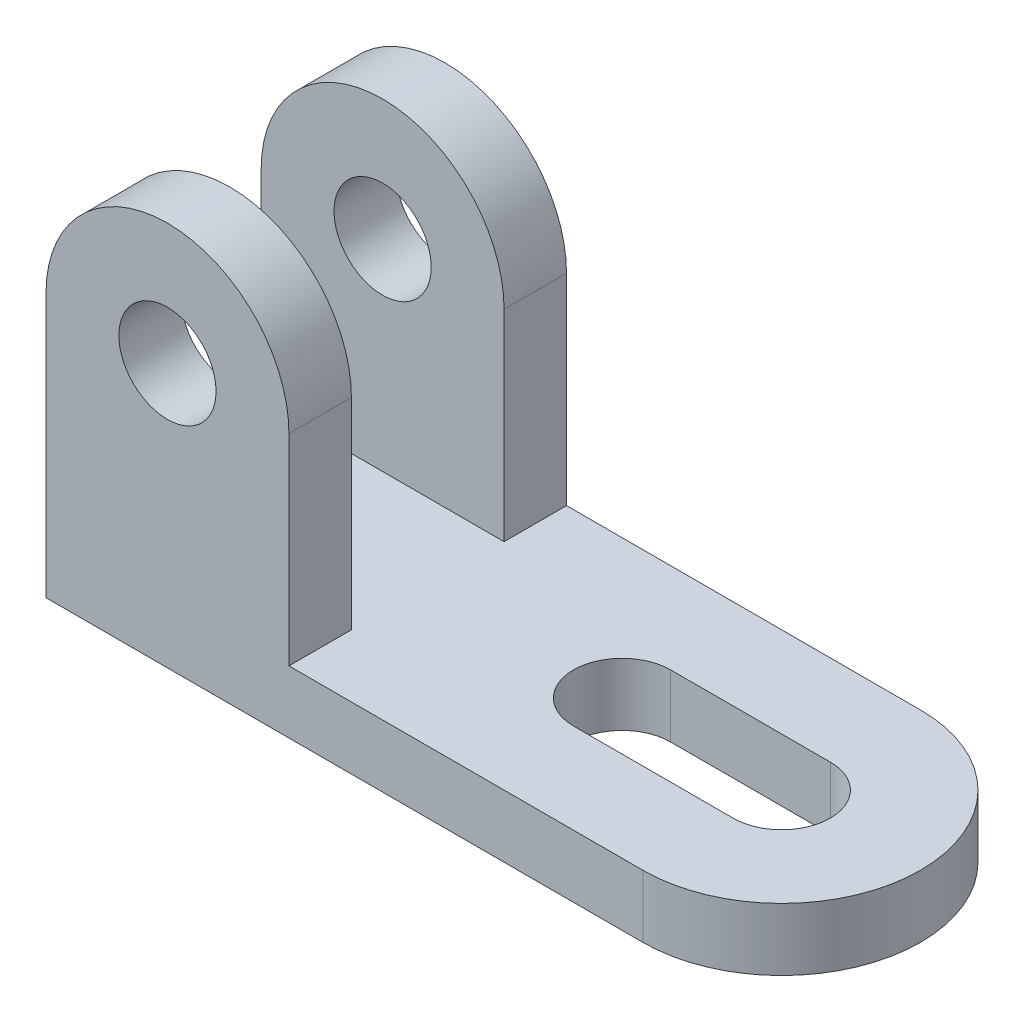
ISO-10303-21;
HEADER;
FILE_DESCRIPTION(('STEP AP214'),'2;1');
FILE_NAME('part.step','',(''),(''),'','','');
FILE_SCHEMA(('AUTOMOTIVE_DESIGN { 1 0 10303 214 1 1 1 1 }'));
ENDSEC;
DATA;
#1=APPLICATION_CONTEXT('core data for automotive mechanical design processes');
#2=APPLICATION_PROTOCOL_DEFINITION('international standard','automotive_design',2000,#1);
#3=PRODUCT_CONTEXT('',#1,'mechanical');
#4=PRODUCT('Part','Part','',(#3));
#5=PRODUCT_RELATED_PRODUCT_CATEGORY('part','',(#4));
#6=PRODUCT_DEFINITION_FORMATION('','',#4);
#7=PRODUCT_DEFINITION_CONTEXT('part definition',#1,'design');
#8=PRODUCT_DEFINITION('design','',#6,#7);
#9=PRODUCT_DEFINITION_SHAPE('','',#8);
#10=(LENGTH_UNIT() NAMED_UNIT(*) SI_UNIT(.MILLI.,.METRE.));
#11=(NAMED_UNIT(*) PLANE_ANGLE_UNIT() SI_UNIT($,.RADIAN.));
#12=(NAMED_UNIT(*) SI_UNIT($,.STERADIAN.) SOLID_ANGLE_UNIT());
#13=UNCERTAINTY_MEASURE_WITH_UNIT(LENGTH_MEASURE(1.E-05),#10,'distance_accuracy_value','');
#14=(GEOMETRIC_REPRESENTATION_CONTEXT(3) GLOBAL_UNCERTAINTY_ASSIGNED_CONTEXT((#13)) GLOBAL_UNIT_ASSIGNED_CONTEXT((#10,
#11,#12)) REPRESENTATION_CONTEXT('',''));
#15=CARTESIAN_POINT('',(0.,0.,0.));
#16=DIRECTION('',(0.,0.,1.));
#17=DIRECTION('',(1.,0.,0.));
#18=AXIS2_PLACEMENT_3D('',#15,#16,#17);
#19=CARTESIAN_POINT('',(86.,9.,0.));
#20=DIRECTION('',(0.,1.,0.));
#21=DIRECTION('',(0.,0.,1.));
#22=AXIS2_PLACEMENT_3D('',#19,#20,#21);
#23=PLANE('',#22);
#24=DIRECTION('',(0.,0.,-1.));
#25=VECTOR('',#24,1.);
#26=CARTESIAN_POINT('',(35.,9.,-11.));
#27=LINE('',#26,#25);
#28=CARTESIAN_POINT('',(35.,9.,-11.));
#29=VERTEX_POINT('',#28);
#30=CARTESIAN_POINT('',(35.,9.,-20.));
#31=VERTEX_POINT('',#30);
#32=EDGE_CURVE('E57',#29,#31,#27,.T.);
#33=ORIENTED_EDGE('',*,*,#32,.F.);
#34=DIRECTION('',(-1.,0.,0.));
#35=VECTOR('',#34,1.);
#36=CARTESIAN_POINT('',(0.,9.,-11.));
#37=LINE('',#36,#35);
#38=CARTESIAN_POINT('',(0.,9.,-11.));
#39=VERTEX_POINT('',#38);
#40=EDGE_CURVE('E164',#29,#39,#37,.T.);
#41=ORIENTED_EDGE('',*,*,#40,.T.);
#42=DIRECTION('',(0.,0.,1.));
#43=VECTOR('',#42,1.);
#44=CARTESIAN_POINT('',(0.,9.,-20.));
#45=LINE('',#44,#43);
#46=CARTESIAN_POINT('',(0.,9.,11.));
#47=VERTEX_POINT('',#46);
#48=EDGE_CURVE('E163',#39,#47,#45,.T.);
#49=ORIENTED_EDGE('',*,*,#48,.T.);
#50=DIRECTION('',(-1.,0.,0.));
#51=VECTOR('',#50,1.);
#52=CARTESIAN_POINT('',(0.,9.,11.));
#53=LINE('',#52,#51);
#54=CARTESIAN_POINT('',(35.,9.,11.));
#55=VERTEX_POINT('',#54);
#56=EDGE_CURVE('E187',#55,#47,#53,.T.);
#57=ORIENTED_EDGE('',*,*,#56,.F.);
#58=DIRECTION('',(0.,0.,1.));
#59=VECTOR('',#58,1.);
#60=CARTESIAN_POINT('',(35.,9.,11.));
#61=LINE('',#60,#59);
#62=CARTESIAN_POINT('',(35.,9.,20.));
#63=VERTEX_POINT('',#62);
#64=EDGE_CURVE('E206',#55,#63,#61,.T.);
#65=ORIENTED_EDGE('',*,*,#64,.T.);
#66=DIRECTION('',(1.,0.,0.));
#67=VECTOR('',#66,1.);
#68=CARTESIAN_POINT('',(86.,9.,20.));
#69=LINE('',#68,#67);
#70=CARTESIAN_POINT('',(86.,9.,20.));
#71=VERTEX_POINT('',#70);
#72=EDGE_CURVE('E241',#63,#71,#69,.T.);
#73=ORIENTED_EDGE('',*,*,#72,.T.);
#74=CARTESIAN_POINT('',(86.,9.,0.));
#75=DIRECTION('',(0.,1.,0.));
#76=DIRECTION('',(0.,0.,1.));
#77=AXIS2_PLACEMENT_3D('',#74,#75,#76);
#78=CIRCLE('',#77,20.);
#79=CARTESIAN_POINT('',(86.,9.,-20.));
#80=VERTEX_POINT('',#79);
#81=EDGE_CURVE('E243',#71,#80,#78,.T.);
#82=ORIENTED_EDGE('',*,*,#81,.T.);
#83=DIRECTION('',(-1.,0.,0.));
#84=VECTOR('',#83,1.);
#85=CARTESIAN_POINT('',(86.,9.,-20.));
#86=LINE('',#85,#84);
#87=EDGE_CURVE('E64',#80,#31,#86,.T.);
#88=ORIENTED_EDGE('',*,*,#87,.T.);
#89=EDGE_LOOP('',(#33,#41,#49,#57,#65,#73,#82,#88));
#90=FACE_BOUND('',#89,.T.);
#91=DIRECTION('',(-1.,0.,0.));
#92=VECTOR('',#91,1.);
#93=CARTESIAN_POINT('',(86.,9.,-7.));
#94=LINE('',#93,#92);
#95=CARTESIAN_POINT('',(86.,9.,-7.));
#96=VERTEX_POINT('',#95);
#97=CARTESIAN_POINT('',(63.,9.,-7.));
#98=VERTEX_POINT('',#97);
#99=EDGE_CURVE('E213',#96,#98,#94,.T.);
#100=ORIENTED_EDGE('',*,*,#99,.F.);
#101=CARTESIAN_POINT('',(86.,9.,0.));
#102=DIRECTION('',(0.,1.,0.));
#103=DIRECTION('',(0.,0.,1.));
#104=AXIS2_PLACEMENT_3D('',#101,#102,#103);
#105=CIRCLE('',#104,7.);
#106=CARTESIAN_POINT('',(86.,9.,7.));
#107=VERTEX_POINT('',#106);
#108=EDGE_CURVE('E211',#107,#96,#105,.T.);
#109=ORIENTED_EDGE('',*,*,#108,.F.);
#110=DIRECTION('',(1.,0.,0.));
#111=VECTOR('',#110,1.);
#112=CARTESIAN_POINT('',(86.,9.,7.));
#113=LINE('',#112,#111);
#114=CARTESIAN_POINT('',(63.,9.,7.));
#115=VERTEX_POINT('',#114);
#116=EDGE_CURVE('E218',#115,#107,#113,.T.);
#117=ORIENTED_EDGE('',*,*,#116,.F.);
#118=CARTESIAN_POINT('',(63.,9.,0.));
#119=DIRECTION('',(0.,1.,0.));
#120=DIRECTION('',(0.,0.,1.));
#121=AXIS2_PLACEMENT_3D('',#118,#119,#120);
#122=CIRCLE('',#121,7.);
#123=EDGE_CURVE('E216',#98,#115,#122,.T.);
#124=ORIENTED_EDGE('',*,*,#123,.F.);
#125=EDGE_LOOP('',(#100,#109,#117,#124));
#126=FACE_BOUND('',#125,.T.);
#127=ADVANCED_FACE('F41',(#90,#126),#23,.T.);
#128=CARTESIAN_POINT('',(86.,0.,0.));
#129=DIRECTION('',(0.,1.,0.));
#130=DIRECTION('',(0.,0.,1.));
#131=AXIS2_PLACEMENT_3D('',#128,#129,#130);
#132=PLANE('',#131);
#133=DIRECTION('',(1.,0.,0.));
#134=VECTOR('',#133,1.);
#135=CARTESIAN_POINT('',(86.,0.,20.));
#136=LINE('',#135,#134);
#137=CARTESIAN_POINT('',(0.,0.,20.));
#138=VERTEX_POINT('',#137);
#139=CARTESIAN_POINT('',(86.,0.,20.));
#140=VERTEX_POINT('',#139);
#141=EDGE_CURVE('E244',#138,#140,#136,.T.);
#142=ORIENTED_EDGE('',*,*,#141,.F.);
#143=DIRECTION('',(0.,0.,1.));
#144=VECTOR('',#143,1.);
#145=CARTESIAN_POINT('',(0.,0.,-20.));
#146=LINE('',#145,#144);
#147=CARTESIAN_POINT('',(0.,0.,-20.));
#148=VERTEX_POINT('',#147);
#149=EDGE_CURVE('E242',#148,#138,#146,.T.);
#150=ORIENTED_EDGE('',*,*,#149,.F.);
#151=DIRECTION('',(-1.,0.,0.));
#152=VECTOR('',#151,1.);
#153=CARTESIAN_POINT('',(86.,0.,-20.));
#154=LINE('',#153,#152);
#155=CARTESIAN_POINT('',(86.,0.,-20.));
#156=VERTEX_POINT('',#155);
#157=EDGE_CURVE('E255',#156,#148,#154,.T.);
#158=ORIENTED_EDGE('',*,*,#157,.F.);
#159=CARTESIAN_POINT('',(86.,0.,0.));
#160=DIRECTION('',(0.,1.,0.));
#161=DIRECTION('',(0.,0.,1.));
#162=AXIS2_PLACEMENT_3D('',#159,#160,#161);
#163=CIRCLE('',#162,20.);
#164=EDGE_CURVE('E252',#140,#156,#163,.T.);
#165=ORIENTED_EDGE('',*,*,#164,.F.);
#166=EDGE_LOOP('',(#142,#150,#158,#165));
#167=FACE_BOUND('',#166,.T.);
#168=CARTESIAN_POINT('',(86.,0.,0.));
#169=DIRECTION('',(0.,1.,0.));
#170=DIRECTION('',(0.,0.,1.));
#171=AXIS2_PLACEMENT_3D('',#168,#169,#170);
#172=CIRCLE('',#171,7.);
#173=CARTESIAN_POINT('',(86.,0.,7.));
#174=VERTEX_POINT('',#173);
#175=CARTESIAN_POINT('',(86.,0.,-7.));
#176=VERTEX_POINT('',#175);
#177=EDGE_CURVE('E202',#174,#176,#172,.T.);
#178=ORIENTED_EDGE('',*,*,#177,.T.);
#179=DIRECTION('',(-1.,0.,0.));
#180=VECTOR('',#179,1.);
#181=CARTESIAN_POINT('',(86.,0.,-7.));
#182=LINE('',#181,#180);
#183=CARTESIAN_POINT('',(63.,0.,-7.));
#184=VERTEX_POINT('',#183);
#185=EDGE_CURVE('E221',#176,#184,#182,.T.);
#186=ORIENTED_EDGE('',*,*,#185,.T.);
#187=CARTESIAN_POINT('',(63.,0.,0.));
#188=DIRECTION('',(0.,1.,0.));
#189=DIRECTION('',(0.,0.,1.));
#190=AXIS2_PLACEMENT_3D('',#187,#188,#189);
#191=CIRCLE('',#190,7.);
#192=CARTESIAN_POINT('',(63.,0.,7.));
#193=VERTEX_POINT('',#192);
#194=EDGE_CURVE('E226',#184,#193,#191,.T.);
#195=ORIENTED_EDGE('',*,*,#194,.T.);
#196=DIRECTION('',(1.,0.,0.));
#197=VECTOR('',#196,1.);
#198=CARTESIAN_POINT('',(86.,0.,7.));
#199=LINE('',#198,#197);
#200=EDGE_CURVE('E212',#193,#174,#199,.T.);
#201=ORIENTED_EDGE('',*,*,#200,.T.);
#202=EDGE_LOOP('',(#178,#186,#195,#201));
#203=FACE_BOUND('',#202,.T.);
#204=ADVANCED_FACE('F271',(#167,#203),#132,.F.);
#205=CARTESIAN_POINT('',(86.,9.,20.));
#206=DIRECTION('',(0.,0.,-1.));
#207=DIRECTION('',(-1.,0.,0.));
#208=AXIS2_PLACEMENT_3D('',#205,#206,#207);
#209=PLANE('',#208);
#210=ORIENTED_EDGE('',*,*,#141,.T.);
#211=DIRECTION('',(0.,-1.,0.));
#212=VECTOR('',#211,1.);
#213=CARTESIAN_POINT('',(86.,9.,20.));
#214=LINE('',#213,#212);
#215=EDGE_CURVE('E11',#71,#140,#214,.T.);
#216=ORIENTED_EDGE('',*,*,#215,.F.);
#217=ORIENTED_EDGE('',*,*,#72,.F.);
#218=DIRECTION('',(0.,-1.,0.));
#219=VECTOR('',#218,1.);
#220=CARTESIAN_POINT('',(35.,0.,20.));
#221=LINE('',#220,#219);
#222=CARTESIAN_POINT('',(35.,38.,20.));
#223=VERTEX_POINT('',#222);
#224=EDGE_CURVE('E183',#223,#63,#221,.T.);
#225=ORIENTED_EDGE('',*,*,#224,.F.);
#226=CARTESIAN_POINT('',(17.5,38.,20.));
#227=DIRECTION('',(0.,0.,1.));
#228=DIRECTION('',(1.,0.,0.));
#229=AXIS2_PLACEMENT_3D('',#226,#227,#228);
#230=CIRCLE('',#229,17.5);
#231=CARTESIAN_POINT('',(0.,38.,20.));
#232=VERTEX_POINT('',#231);
#233=EDGE_CURVE('E196',#232,#223,#230,.F.);
#234=ORIENTED_EDGE('',*,*,#233,.F.);
#235=DIRECTION('',(0.,-1.,0.));
#236=VECTOR('',#235,1.);
#237=CARTESIAN_POINT('',(0.,9.,20.));
#238=LINE('',#237,#236);
#239=EDGE_CURVE('E247',#232,#138,#238,.T.);
#240=ORIENTED_EDGE('',*,*,#239,.T.);
#241=EDGE_LOOP('',(#210,#216,#217,#225,#234,#240));
#242=FACE_BOUND('',#241,.T.);
#243=CARTESIAN_POINT('',(17.5,38.,20.));
#244=DIRECTION('',(0.,0.,1.));
#245=DIRECTION('',(1.,0.,0.));
#246=AXIS2_PLACEMENT_3D('',#243,#244,#245);
#247=CIRCLE('',#246,7.);
#248=CARTESIAN_POINT('',(24.5,38.,20.));
#249=VERTEX_POINT('',#248);
#250=EDGE_CURVE('E155',#249,#249,#247,.T.);
#251=ORIENTED_EDGE('',*,*,#250,.F.);
#252=EDGE_LOOP('',(#251));
#253=FACE_BOUND('',#252,.T.);
#254=ADVANCED_FACE('F43',(#242,#253),#209,.F.);
#255=CARTESIAN_POINT('',(86.,9.,0.));
#256=DIRECTION('',(0.,-1.,0.));
#257=DIRECTION('',(0.,0.,-1.));
#258=AXIS2_PLACEMENT_3D('',#255,#256,#257);
#259=CYLINDRICAL_SURFACE('',#258,20.);
#260=ORIENTED_EDGE('',*,*,#164,.T.);
#261=DIRECTION('',(0.,-1.,0.));
#262=VECTOR('',#261,1.);
#263=CARTESIAN_POINT('',(86.,9.,-20.));
#264=LINE('',#263,#262);
#265=EDGE_CURVE('E47',#80,#156,#264,.T.);
#266=ORIENTED_EDGE('',*,*,#265,.F.);
#267=ORIENTED_EDGE('',*,*,#81,.F.);
#268=ORIENTED_EDGE('',*,*,#215,.T.);
#269=EDGE_LOOP('',(#260,#266,#267,#268));
#270=FACE_BOUND('',#269,.T.);
#271=ADVANCED_FACE('F320',(#270),#259,.T.);
#272=CARTESIAN_POINT('',(86.,9.,-20.));
#273=DIRECTION('',(0.,0.,1.));
#274=DIRECTION('',(1.,0.,0.));
#275=AXIS2_PLACEMENT_3D('',#272,#273,#274);
#276=PLANE('',#275);
#277=ORIENTED_EDGE('',*,*,#157,.T.);
#278=DIRECTION('',(0.,-1.,0.));
#279=VECTOR('',#278,1.);
#280=CARTESIAN_POINT('',(0.,9.,-20.));
#281=LINE('',#280,#279);
#282=CARTESIAN_POINT('',(0.,38.,-20.));
#283=VERTEX_POINT('',#282);
#284=EDGE_CURVE('E259',#283,#148,#281,.T.);
#285=ORIENTED_EDGE('',*,*,#284,.F.);
#286=CARTESIAN_POINT('',(17.5,38.,-20.));
#287=DIRECTION('',(0.,0.,1.));
#288=DIRECTION('',(1.,0.,0.));
#289=AXIS2_PLACEMENT_3D('',#286,#287,#288);
#290=CIRCLE('',#289,17.5);
#291=CARTESIAN_POINT('',(35.,38.,-20.));
#292=VERTEX_POINT('',#291);
#293=EDGE_CURVE('E146',#283,#292,#290,.F.);
#294=ORIENTED_EDGE('',*,*,#293,.T.);
#295=DIRECTION('',(0.,-1.,0.));
#296=VECTOR('',#295,1.);
#297=CARTESIAN_POINT('',(35.,0.,-20.));
#298=LINE('',#297,#296);
#299=EDGE_CURVE('E176',#292,#31,#298,.T.);
#300=ORIENTED_EDGE('',*,*,#299,.T.);
#301=ORIENTED_EDGE('',*,*,#87,.F.);
#302=ORIENTED_EDGE('',*,*,#265,.T.);
#303=EDGE_LOOP('',(#277,#285,#294,#300,#301,#302));
#304=FACE_BOUND('',#303,.T.);
#305=CARTESIAN_POINT('',(17.5,38.,-20.));
#306=DIRECTION('',(0.,0.,1.));
#307=DIRECTION('',(1.,0.,0.));
#308=AXIS2_PLACEMENT_3D('',#305,#306,#307);
#309=CIRCLE('',#308,7.);
#310=CARTESIAN_POINT('',(24.5,38.,-20.));
#311=VERTEX_POINT('',#310);
#312=EDGE_CURVE('E171',#311,#311,#309,.T.);
#313=ORIENTED_EDGE('',*,*,#312,.T.);
#314=EDGE_LOOP('',(#313));
#315=FACE_BOUND('',#314,.T.);
#316=ADVANCED_FACE('F262',(#304,#315),#276,.F.);
#317=CARTESIAN_POINT('',(0.,9.,-20.));
#318=DIRECTION('',(1.,0.,0.));
#319=DIRECTION('',(0.,0.,-1.));
#320=AXIS2_PLACEMENT_3D('',#317,#318,#319);
#321=PLANE('',#320);
#322=ORIENTED_EDGE('',*,*,#149,.T.);
#323=ORIENTED_EDGE('',*,*,#239,.F.);
#324=DIRECTION('',(0.,0.,1.));
#325=VECTOR('',#324,1.);
#326=CARTESIAN_POINT('',(0.,38.,11.));
#327=LINE('',#326,#325);
#328=CARTESIAN_POINT('',(0.,38.,11.));
#329=VERTEX_POINT('',#328);
#330=EDGE_CURVE('E194',#329,#232,#327,.T.);
#331=ORIENTED_EDGE('',*,*,#330,.F.);
#332=DIRECTION('',(0.,1.,0.));
#333=VECTOR('',#332,1.);
#334=CARTESIAN_POINT('',(0.,0.,11.));
#335=LINE('',#334,#333);
#336=EDGE_CURVE('E190',#47,#329,#335,.T.);
#337=ORIENTED_EDGE('',*,*,#336,.F.);
#338=ORIENTED_EDGE('',*,*,#48,.F.);
#339=DIRECTION('',(0.,1.,0.));
#340=VECTOR('',#339,1.);
#341=CARTESIAN_POINT('',(0.,0.,-11.));
#342=LINE('',#341,#340);
#343=CARTESIAN_POINT('',(0.,38.,-11.));
#344=VERTEX_POINT('',#343);
#345=EDGE_CURVE('E160',#39,#344,#342,.T.);
#346=ORIENTED_EDGE('',*,*,#345,.T.);
#347=DIRECTION('',(0.,0.,-1.));
#348=VECTOR('',#347,1.);
#349=CARTESIAN_POINT('',(0.,38.,-11.));
#350=LINE('',#349,#348);
#351=EDGE_CURVE('E142',#344,#283,#350,.T.);
#352=ORIENTED_EDGE('',*,*,#351,.T.);
#353=ORIENTED_EDGE('',*,*,#284,.T.);
#354=EDGE_LOOP('',(#322,#323,#331,#337,#338,#346,#352,#353));
#355=FACE_BOUND('',#354,.T.);
#356=ADVANCED_FACE('F165',(#355),#321,.F.);
#357=CARTESIAN_POINT('',(86.,9.,0.));
#358=DIRECTION('',(0.,-1.,0.));
#359=DIRECTION('',(0.,0.,-1.));
#360=AXIS2_PLACEMENT_3D('',#357,#358,#359);
#361=CYLINDRICAL_SURFACE('',#360,7.);
#362=ORIENTED_EDGE('',*,*,#177,.F.);
#363=DIRECTION('',(0.,-1.,0.));
#364=VECTOR('',#363,1.);
#365=CARTESIAN_POINT('',(86.,9.,7.));
#366=LINE('',#365,#364);
#367=EDGE_CURVE('E222',#107,#174,#366,.T.);
#368=ORIENTED_EDGE('',*,*,#367,.F.);
#369=ORIENTED_EDGE('',*,*,#108,.T.);
#370=DIRECTION('',(0.,-1.,0.));
#371=VECTOR('',#370,1.);
#372=CARTESIAN_POINT('',(86.,9.,-7.));
#373=LINE('',#372,#371);
#374=EDGE_CURVE('E236',#96,#176,#373,.T.);
#375=ORIENTED_EDGE('',*,*,#374,.T.);
#376=EDGE_LOOP('',(#362,#368,#369,#375));
#377=FACE_BOUND('',#376,.T.);
#378=ADVANCED_FACE('F315',(#377),#361,.F.);
#379=CARTESIAN_POINT('',(86.,9.,-7.));
#380=DIRECTION('',(0.,0.,1.));
#381=DIRECTION('',(1.,0.,0.));
#382=AXIS2_PLACEMENT_3D('',#379,#380,#381);
#383=PLANE('',#382);
#384=ORIENTED_EDGE('',*,*,#185,.F.);
#385=ORIENTED_EDGE('',*,*,#374,.F.);
#386=ORIENTED_EDGE('',*,*,#99,.T.);
#387=DIRECTION('',(0.,-1.,0.));
#388=VECTOR('',#387,1.);
#389=CARTESIAN_POINT('',(63.,9.,-7.));
#390=LINE('',#389,#388);
#391=EDGE_CURVE('E237',#98,#184,#390,.T.);
#392=ORIENTED_EDGE('',*,*,#391,.T.);
#393=EDGE_LOOP('',(#384,#385,#386,#392));
#394=FACE_BOUND('',#393,.T.);
#395=ADVANCED_FACE('F408',(#394),#383,.T.);
#396=CARTESIAN_POINT('',(63.,9.,0.));
#397=DIRECTION('',(0.,-1.,0.));
#398=DIRECTION('',(0.,0.,-1.));
#399=AXIS2_PLACEMENT_3D('',#396,#397,#398);
#400=CYLINDRICAL_SURFACE('',#399,7.);
#401=ORIENTED_EDGE('',*,*,#194,.F.);
#402=ORIENTED_EDGE('',*,*,#391,.F.);
#403=ORIENTED_EDGE('',*,*,#123,.T.);
#404=DIRECTION('',(0.,-1.,0.));
#405=VECTOR('',#404,1.);
#406=CARTESIAN_POINT('',(63.,9.,7.));
#407=LINE('',#406,#405);
#408=EDGE_CURVE('E232',#115,#193,#407,.T.);
#409=ORIENTED_EDGE('',*,*,#408,.T.);
#410=EDGE_LOOP('',(#401,#402,#403,#409));
#411=FACE_BOUND('',#410,.T.);
#412=ADVANCED_FACE('F406',(#411),#400,.F.);
#413=CARTESIAN_POINT('',(86.,9.,7.));
#414=DIRECTION('',(0.,0.,-1.));
#415=DIRECTION('',(-1.,0.,0.));
#416=AXIS2_PLACEMENT_3D('',#413,#414,#415);
#417=PLANE('',#416);
#418=ORIENTED_EDGE('',*,*,#200,.F.);
#419=ORIENTED_EDGE('',*,*,#408,.F.);
#420=ORIENTED_EDGE('',*,*,#116,.T.);
#421=ORIENTED_EDGE('',*,*,#367,.T.);
#422=EDGE_LOOP('',(#418,#419,#420,#421));
#423=FACE_BOUND('',#422,.T.);
#424=ADVANCED_FACE('F335',(#423),#417,.T.);
#425=CARTESIAN_POINT('',(17.5,38.,11.));
#426=DIRECTION('',(0.,0.,1.));
#427=DIRECTION('',(1.,0.,0.));
#428=AXIS2_PLACEMENT_3D('',#425,#426,#427);
#429=CYLINDRICAL_SURFACE('',#428,17.5);
#430=ORIENTED_EDGE('',*,*,#233,.T.);
#431=DIRECTION('',(0.,0.,1.));
#432=VECTOR('',#431,1.);
#433=CARTESIAN_POINT('',(35.,38.,11.));
#434=LINE('',#433,#432);
#435=CARTESIAN_POINT('',(35.,38.,11.));
#436=VERTEX_POINT('',#435);
#437=EDGE_CURVE('E205',#436,#223,#434,.T.);
#438=ORIENTED_EDGE('',*,*,#437,.F.);
#439=CARTESIAN_POINT('',(17.5,38.,11.));
#440=DIRECTION('',(0.,0.,1.));
#441=DIRECTION('',(1.,0.,0.));
#442=AXIS2_PLACEMENT_3D('',#439,#440,#441);
#443=CIRCLE('',#442,17.5);
#444=EDGE_CURVE('E184',#329,#436,#443,.F.);
#445=ORIENTED_EDGE('',*,*,#444,.F.);
#446=ORIENTED_EDGE('',*,*,#330,.T.);
#447=EDGE_LOOP('',(#430,#438,#445,#446));
#448=FACE_BOUND('',#447,.T.);
#449=ADVANCED_FACE('F284',(#448),#429,.T.);
#450=CARTESIAN_POINT('',(35.,0.,11.));
#451=DIRECTION('',(-1.,0.,0.));
#452=DIRECTION('',(0.,-1.,0.));
#453=AXIS2_PLACEMENT_3D('',#450,#451,#452);
#454=PLANE('',#453);
#455=ORIENTED_EDGE('',*,*,#224,.T.);
#456=ORIENTED_EDGE('',*,*,#64,.F.);
#457=DIRECTION('',(0.,-1.,0.));
#458=VECTOR('',#457,1.);
#459=CARTESIAN_POINT('',(35.,0.,11.));
#460=LINE('',#459,#458);
#461=EDGE_CURVE('E193',#436,#55,#460,.T.);
#462=ORIENTED_EDGE('',*,*,#461,.F.);
#463=ORIENTED_EDGE('',*,*,#437,.T.);
#464=EDGE_LOOP('',(#455,#456,#462,#463));
#465=FACE_BOUND('',#464,.T.);
#466=ADVANCED_FACE('F340',(#465),#454,.F.);
#467=CARTESIAN_POINT('',(17.5,38.,11.));
#468=DIRECTION('',(0.,0.,1.));
#469=DIRECTION('',(1.,0.,0.));
#470=AXIS2_PLACEMENT_3D('',#467,#468,#469);
#471=CYLINDRICAL_SURFACE('',#470,7.);
#472=CARTESIAN_POINT('',(17.5,38.,11.));
#473=DIRECTION('',(0.,0.,1.));
#474=DIRECTION('',(1.,0.,0.));
#475=AXIS2_PLACEMENT_3D('',#472,#473,#474);
#476=CIRCLE('',#475,7.);
#477=CARTESIAN_POINT('',(24.5,38.,11.));
#478=VERTEX_POINT('',#477);
#479=EDGE_CURVE('E182',#478,#478,#476,.T.);
#480=ORIENTED_EDGE('',*,*,#479,.F.);
#481=EDGE_LOOP('',(#480));
#482=FACE_BOUND('',#481,.T.);
#483=ORIENTED_EDGE('',*,*,#250,.T.);
#484=EDGE_LOOP('',(#483));
#485=FACE_BOUND('',#484,.T.);
#486=ADVANCED_FACE('F347',(#482,#485),#471,.F.);
#487=CARTESIAN_POINT('',(0.,0.,11.));
#488=DIRECTION('',(0.,0.,1.));
#489=DIRECTION('',(1.,0.,0.));
#490=AXIS2_PLACEMENT_3D('',#487,#488,#489);
#491=PLANE('',#490);
#492=ORIENTED_EDGE('',*,*,#479,.T.);
#493=EDGE_LOOP('',(#492));
#494=FACE_BOUND('',#493,.T.);
#495=ORIENTED_EDGE('',*,*,#444,.T.);
#496=ORIENTED_EDGE('',*,*,#461,.T.);
#497=ORIENTED_EDGE('',*,*,#56,.T.);
#498=ORIENTED_EDGE('',*,*,#336,.T.);
#499=EDGE_LOOP('',(#495,#496,#497,#498));
#500=FACE_BOUND('',#499,.T.);
#501=ADVANCED_FACE('F283',(#494,#500),#491,.F.);
#502=CARTESIAN_POINT('',(17.5,38.,-11.));
#503=DIRECTION('',(0.,0.,-1.));
#504=DIRECTION('',(-1.,0.,0.));
#505=AXIS2_PLACEMENT_3D('',#502,#503,#504);
#506=CYLINDRICAL_SURFACE('',#505,17.5);
#507=ORIENTED_EDGE('',*,*,#293,.F.);
#508=ORIENTED_EDGE('',*,*,#351,.F.);
#509=CARTESIAN_POINT('',(17.5,38.,-11.));
#510=DIRECTION('',(0.,0.,1.));
#511=DIRECTION('',(1.,0.,0.));
#512=AXIS2_PLACEMENT_3D('',#509,#510,#511);
#513=CIRCLE('',#512,17.5);
#514=CARTESIAN_POINT('',(35.,38.,-11.));
#515=VERTEX_POINT('',#514);
#516=EDGE_CURVE('E144',#344,#515,#513,.F.);
#517=ORIENTED_EDGE('',*,*,#516,.T.);
#518=DIRECTION('',(0.,0.,-1.));
#519=VECTOR('',#518,1.);
#520=CARTESIAN_POINT('',(35.,38.,-11.));
#521=LINE('',#520,#519);
#522=EDGE_CURVE('E174',#515,#292,#521,.T.);
#523=ORIENTED_EDGE('',*,*,#522,.T.);
#524=EDGE_LOOP('',(#507,#508,#517,#523));
#525=FACE_BOUND('',#524,.T.);
#526=ADVANCED_FACE('F145',(#525),#506,.T.);
#527=CARTESIAN_POINT('',(17.5,38.,-11.));
#528=DIRECTION('',(0.,0.,-1.));
#529=DIRECTION('',(-1.,0.,0.));
#530=AXIS2_PLACEMENT_3D('',#527,#528,#529);
#531=CYLINDRICAL_SURFACE('',#530,7.);
#532=CARTESIAN_POINT('',(17.5,38.,-11.));
#533=DIRECTION('',(0.,0.,1.));
#534=DIRECTION('',(1.,0.,0.));
#535=AXIS2_PLACEMENT_3D('',#532,#533,#534);
#536=CIRCLE('',#535,7.);
#537=CARTESIAN_POINT('',(24.5,38.,-11.));
#538=VERTEX_POINT('',#537);
#539=EDGE_CURVE('E159',#538,#538,#536,.T.);
#540=ORIENTED_EDGE('',*,*,#539,.T.);
#541=EDGE_LOOP('',(#540));
#542=FACE_BOUND('',#541,.T.);
#543=ORIENTED_EDGE('',*,*,#312,.F.);
#544=EDGE_LOOP('',(#543));
#545=FACE_BOUND('',#544,.T.);
#546=ADVANCED_FACE('F295',(#542,#545),#531,.F.);
#547=CARTESIAN_POINT('',(35.,0.,-11.));
#548=DIRECTION('',(1.,0.,0.));
#549=DIRECTION('',(0.,1.,0.));
#550=AXIS2_PLACEMENT_3D('',#547,#548,#549);
#551=PLANE('',#550);
#552=ORIENTED_EDGE('',*,*,#299,.F.);
#553=ORIENTED_EDGE('',*,*,#522,.F.);
#554=DIRECTION('',(0.,-1.,0.));
#555=VECTOR('',#554,1.);
#556=CARTESIAN_POINT('',(35.,0.,-11.));
#557=LINE('',#556,#555);
#558=EDGE_CURVE('E157',#515,#29,#557,.T.);
#559=ORIENTED_EDGE('',*,*,#558,.T.);
#560=ORIENTED_EDGE('',*,*,#32,.T.);
#561=EDGE_LOOP('',(#552,#553,#559,#560));
#562=FACE_BOUND('',#561,.T.);
#563=ADVANCED_FACE('F289',(#562),#551,.T.);
#564=CARTESIAN_POINT('',(0.,0.,-11.));
#565=DIRECTION('',(0.,0.,1.));
#566=DIRECTION('',(1.,0.,0.));
#567=AXIS2_PLACEMENT_3D('',#564,#565,#566);
#568=PLANE('',#567);
#569=ORIENTED_EDGE('',*,*,#539,.F.);
#570=EDGE_LOOP('',(#569));
#571=FACE_BOUND('',#570,.T.);
#572=ORIENTED_EDGE('',*,*,#516,.F.);
#573=ORIENTED_EDGE('',*,*,#345,.F.);
#574=ORIENTED_EDGE('',*,*,#40,.F.);
#575=ORIENTED_EDGE('',*,*,#558,.F.);
#576=EDGE_LOOP('',(#572,#573,#574,#575));
#577=FACE_BOUND('',#576,.T.);
#578=ADVANCED_FACE('F156',(#571,#577),#568,.T.);
#579=CLOSED_SHELL('',(#127,#204,#254,#271,#316,#356,#378,#395,#412,#424,#449,#466,#486,#501,
#526,#546,#563,#578));
#580=MANIFOLD_SOLID_BREP('B2',#579);
#581=ADVANCED_BREP_SHAPE_REPRESENTATION('',(#18,#580),#14);
#582=SHAPE_DEFINITION_REPRESENTATION(#9,#581);
ENDSEC;
END-ISO-10303-21;
